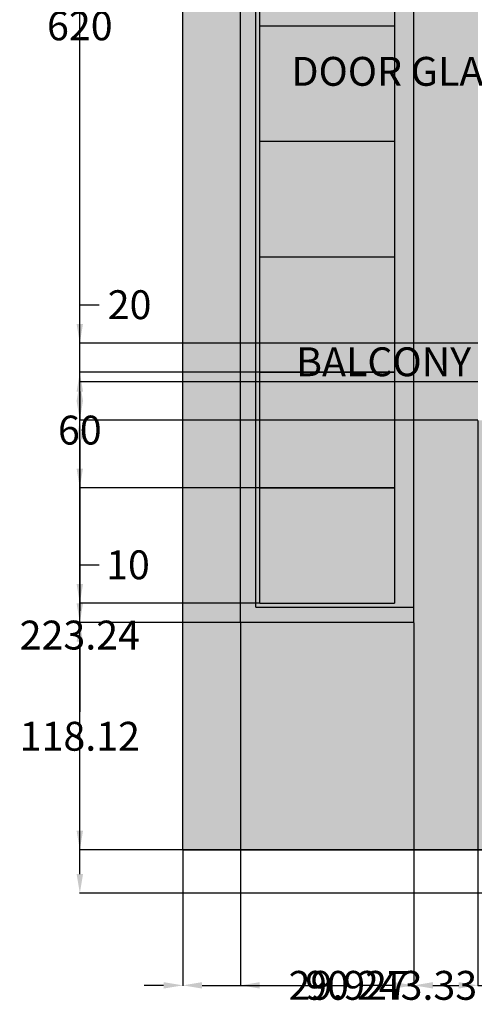
# Model space of a CAD drawing. Units: millimetres. Extents: x 131 to 845, y -20 to 1043.
# Tile 1 of 11: x 131 to 368, y -20 to 492. Entities that reach past the tile are written whole.
import ezdxf

# ---------------------------------------------------------------- set-up
doc = ezdxf.new("R2010")
doc.units = ezdxf.units.MM
doc.header["$MEASUREMENT"] = 0
for name, color, linetype, lineweight in [('A-ANNO-DIMS', 2, 'Continuous', 18), ('A-ELEV', 7, 'Continuous', 25), ('A-ELEV-PATT', 7, 'Continuous', 13), ('A-GLAZ', 4, 'Continuous', 25), ('A-WALL-PATT', 131, 'Continuous', 13)]:
    doc.layers.add(name, color=color, linetype=linetype, lineweight=lineweight)
doc.styles.get("Standard").update_dxf_attribs({"font": 'arial.ttf'})
doc.dimstyles.get("Standard").update_dxf_attribs({"dimtxt": 15, "dimasz": 10, "dimexe": 0.18, "dimexo": 0.0625, "dimgap": 5, "dimtad": 0, "dimtih": 1, "dimtoh": 1, "dimdec": 0, "dimzin": 0, "dimdsep": 46, "dimtxsty": 'Standard', "dimcen": 5, "dimadec": 0, "dimazin": 0, "dimtfac": 1, "dimtdec": 0, "dimtofl": 0, "dimtmove": 0, "dimatfit": 3, "dimfxl": 1, "dimtolj": 1, "dimtzin": 0, "dimarcsym": 0})

# ---------------------------------------------------------------- blocks, each defined once
blk = doc.blocks.new('*U3')
blk.add_line((0, -70), (0, 0))
blk = doc.blocks.new('*U4')
at = {"layer": 'A-GLAZ', "color": 0, "linetype": 'ByBlock', "lineweight": -2, "transparency": 16777216, "rotation": 270}
for p in [(326.16, 488.43), (326.16, 428.43), (326.16, 368.43), (326.16, 308.43), (326.16, 248.43), (326.16, 188.43)]:
    blk.add_blockref('*U3', p, dxfattribs=at)
blk = doc.blocks.new('*D9')
at = {"layer": 'A-ANNO-DIMS', "color": 0, "lineweight": -2, "transparency": 16777216}
for p, q in [((571.05, 313.91), (561.05, 313.91)), ((581.05, 313.22), (581.05, 314.09)), ((586.05, 313.22), (586.05, 314.09)), ((596.05, 313.91), (606.05, 313.91))]:
    blk.add_line(p, q, dxfattribs=at)
at = {"layer": 'A-ANNO-DIMS', "color": 0, "transparency": 16777216}
for points in [[(571.05, 315.58), (571.05, 312.24), (581.05, 313.91)], [(596.05, 315.58), (596.05, 312.24), (586.05, 313.91)]]:
    blk.add_solid(points, dxfattribs=at)
at = {"layer": 'Defpoints', "color": 0, "transparency": 16777216}
for p in [(581.05, 313.91), (581.05, 313.16), (586.05, 313.16)]:
    blk.add_point(p, dxfattribs=at)
at = {"layer": 'A-ANNO-DIMS', "color": 0, "transparency": 16777216, "insert": (409.24, 313.91), "char_height": 15, "attachment_point": 5}
blk.add_mtext('\\A1;BALCONY RAIL PANEL 5 TYP.', dxfattribs=at)
blk = doc.blocks.new('*D11')
at = {"layer": 'A-ANNO-DIMS', "color": 0, "lineweight": -2, "transparency": 16777216}
for p, q in [((554.73, 464.78), (544.73, 464.78)), ((554.75, 454.78), (554.73, 464.78)), ((550.09, 454.77), (554.93, 454.78)), ((554.78, 433.28), (554.76, 444.78)), ((550.13, 423.27), (554.97, 423.28))]:
    blk.add_line(p, q, dxfattribs=at)
at = {"layer": 'A-ANNO-DIMS', "color": 0, "transparency": 16777216}
for points in [[(556.43, 444.78), (553.1, 444.77), (554.75, 454.78)], [(556.45, 433.28), (553.11, 433.27), (554.79, 423.28)]]:
    blk.add_solid(points, dxfattribs=at)
at = {"layer": 'Defpoints', "color": 0, "transparency": 16777216}
for p in [(550.02, 454.77), (554.75, 454.78), (550.07, 423.27)]:
    blk.add_point(p, dxfattribs=at)
at = {"layer": 'A-ANNO-DIMS', "color": 0, "transparency": 16777216, "insert": (399.96, 464.78), "char_height": 15, "attachment_point": 5}
blk.add_mtext('\\A1;DOOR GLASS PANE 32 TYP.', dxfattribs=at)
blk = doc.blocks.new('*D14')
at = {"layer": 'A-ANNO-DIMS', "color": 0, "lineweight": -2, "transparency": 16777216}
for p, q in [((210.52, 985.67), (162.55, 985.67)), ((162.73, 975.67), (162.73, 524.4)), ((162.73, 47.81), (162.73, 499.08)), ((459.5, 37.81), (162.55, 37.81))]:
    blk.add_line(p, q, dxfattribs=at)
at = {"layer": 'A-ANNO-DIMS', "color": 0, "transparency": 16777216}
for points in [[(161.06, 975.67), (164.4, 975.67), (162.73, 985.67)], [(161.06, 47.81), (164.4, 47.81), (162.73, 37.81)]]:
    blk.add_solid(points, dxfattribs=at)
at = {"layer": 'Defpoints', "color": 0, "transparency": 16777216}
for p in [(162.73, 985.67), (210.58, 985.67), (459.56, 37.81)]:
    blk.add_point(p, dxfattribs=at)
at = {"layer": 'A-ANNO-DIMS', "color": 0, "transparency": 16777216, "insert": (162.73, 511.74), "char_height": 15, "attachment_point": 5}
blk.add_mtext('\\A1;947.9', dxfattribs=at)
blk = doc.blocks.new('*D17')
at = {"layer": 'A-ANNO-DIMS', "color": 0, "lineweight": -2, "transparency": 16777216}
for p, q in [((216.17, 960.67), (162.55, 960.67)), ((162.73, 950.67), (162.73, 523.15)), ((162.73, 70.31), (162.73, 497.83)), ((216.17, 60.31), (162.55, 60.31))]:
    blk.add_line(p, q, dxfattribs=at)
at = {"layer": 'A-ANNO-DIMS', "color": 0, "transparency": 16777216}
for points in [[(161.06, 950.67), (164.4, 950.67), (162.73, 960.67)], [(161.06, 70.31), (164.4, 70.31), (162.73, 60.31)]]:
    blk.add_solid(points, dxfattribs=at)
at = {"layer": 'Defpoints', "color": 0, "transparency": 16777216}
for p in [(162.73, 960.67), (216.23, 960.67), (216.23, 60.31)]:
    blk.add_point(p, dxfattribs=at)
at = {"layer": 'A-ANNO-DIMS', "color": 0, "transparency": 16777216, "insert": (162.73, 510.49), "char_height": 15, "attachment_point": 5}
blk.add_mtext('\\A1;900.4', dxfattribs=at)
blk = doc.blocks.new('*D18')
at = {"layer": 'A-ANNO-DIMS', "color": 0, "lineweight": -2, "transparency": 16777216}
for p, q in [((216.23, 60.25), (216.23, -10.22)), ((459.56, 60.25), (459.56, -10.22)), ((226.23, -10.04), (301.63, -10.04)), ((449.56, -10.04), (374.16, -10.04))]:
    blk.add_line(p, q, dxfattribs=at)
at = {"layer": 'A-ANNO-DIMS', "color": 0, "transparency": 16777216}
for points in [[(226.23, -8.37), (226.23, -11.7), (216.23, -10.04)], [(449.56, -8.37), (449.56, -11.7), (459.56, -10.04)]]:
    blk.add_solid(points, dxfattribs=at)
at = {"layer": 'Defpoints', "color": 0, "transparency": 16777216}
for p in [(216.23, 60.31), (459.56, 60.31), (459.56, -10.04)]:
    blk.add_point(p, dxfattribs=at)
at = {"layer": 'A-ANNO-DIMS', "color": 0, "transparency": 16777216, "insert": (337.9, -10.04), "char_height": 15, "attachment_point": 5}
blk.add_mtext('\\A1;243.33', dxfattribs=at)
blk = doc.blocks.new('*D25')
at = {"layer": 'A-ANNO-DIMS', "color": 0, "lineweight": -2, "transparency": 16777216}
for p, q in [((246.16, 178.37), (246.16, -10.22)), ((216.23, 60.25), (216.23, -10.22)), ((206.23, -10.04), (196.23, -10.04)), ((256.16, -10.04), (266.16, -10.04))]:
    blk.add_line(p, q, dxfattribs=at)
at = {"layer": 'A-ANNO-DIMS', "color": 0, "transparency": 16777216}
for points in [[(206.23, -8.37), (206.23, -11.7), (216.23, -10.04)], [(256.16, -8.37), (256.16, -11.7), (246.16, -10.04)]]:
    blk.add_solid(points, dxfattribs=at)
at = {"layer": 'Defpoints', "color": 0, "transparency": 16777216}
for p in [(246.16, 178.43), (216.23, 60.31), (246.16, -10.04)]:
    blk.add_point(p, dxfattribs=at)
at = {"layer": 'A-ANNO-DIMS', "color": 0, "transparency": 16777216, "insert": (302.42, -10.04), "char_height": 15, "attachment_point": 5}
blk.add_mtext('\\A1;29.927', dxfattribs=at)
blk = doc.blocks.new('*D26')
at = {"layer": 'A-ANNO-DIMS', "color": 0, "lineweight": -2, "transparency": 16777216}
for p, q in [((246.16, 178.37), (246.16, -10.22)), ((336.16, 178.37), (336.16, -10.22)), ((256.16, -10.04), (275.44, -10.04)), ((326.16, -10.04), (306.88, -10.04))]:
    blk.add_line(p, q, dxfattribs=at)
at = {"layer": 'A-ANNO-DIMS', "color": 0, "transparency": 16777216}
for points in [[(256.16, -8.37), (256.16, -11.7), (246.16, -10.04)], [(326.16, -8.37), (326.16, -11.7), (336.16, -10.04)]]:
    blk.add_solid(points, dxfattribs=at)
at = {"layer": 'Defpoints', "color": 0, "transparency": 16777216}
for p in [(246.16, 178.43), (336.16, 178.43), (336.16, -10.04)]:
    blk.add_point(p, dxfattribs=at)
at = {"layer": 'A-ANNO-DIMS', "color": 0, "transparency": 16777216, "insert": (291.16, -10.04), "char_height": 15, "attachment_point": 5}
blk.add_mtext('\\A1;90', dxfattribs=at)
blk = doc.blocks.new('*D27')
at = {"layer": 'A-ANNO-DIMS', "color": 0, "lineweight": -2, "transparency": 16777216}
for p, q in [((246.1, 178.43), (162.55, 178.43)), ((162.73, 168.43), (162.73, 132.03)), ((162.73, 70.31), (162.73, 106.71)), ((216.17, 60.31), (162.55, 60.31))]:
    blk.add_line(p, q, dxfattribs=at)
at = {"layer": 'A-ANNO-DIMS', "color": 0, "transparency": 16777216}
for points in [[(161.06, 168.43), (164.4, 168.43), (162.73, 178.43)], [(161.06, 70.31), (164.4, 70.31), (162.73, 60.31)]]:
    blk.add_solid(points, dxfattribs=at)
at = {"layer": 'Defpoints', "color": 0, "transparency": 16777216}
for p in [(246.16, 178.43), (162.73, 60.31), (216.23, 60.31)]:
    blk.add_point(p, dxfattribs=at)
at = {"layer": 'A-ANNO-DIMS', "color": 0, "transparency": 16777216, "insert": (162.73, 119.37), "char_height": 15, "attachment_point": 5}
blk.add_mtext('\\A1;118.12', dxfattribs=at)
blk = doc.blocks.new('*D28')
at = {"layer": 'A-ANNO-DIMS', "color": 0, "lineweight": -2, "transparency": 16777216}
for p, q in [((246.1, 798.43), (162.55, 798.43)), ((162.73, 788.43), (162.73, 501.09)), ((162.73, 188.43), (162.73, 475.77)), ((246.1, 178.43), (162.55, 178.43))]:
    blk.add_line(p, q, dxfattribs=at)
at = {"layer": 'A-ANNO-DIMS', "color": 0, "transparency": 16777216}
for points in [[(161.06, 788.43), (164.4, 788.43), (162.73, 798.43)], [(161.06, 188.43), (164.4, 188.43), (162.73, 178.43)]]:
    blk.add_solid(points, dxfattribs=at)
at = {"layer": 'Defpoints', "color": 0, "transparency": 16777216}
for p in [(162.73, 798.43), (246.16, 798.43), (246.16, 178.43)]:
    blk.add_point(p, dxfattribs=at)
at = {"layer": 'A-ANNO-DIMS', "color": 0, "transparency": 16777216, "insert": (162.73, 488.43), "char_height": 15, "attachment_point": 5}
blk.add_mtext('\\A1;620', dxfattribs=at)
blk = doc.blocks.new('*D29')
at = {"layer": 'A-ANNO-DIMS', "color": 0, "lineweight": -2, "transparency": 16777216}
for p, q in [((326.1, 308.43), (162.55, 308.43)), ((162.73, 298.43), (162.73, 291.09)), ((162.73, 258.43), (162.73, 265.77)), ((326.1, 248.43), (162.55, 248.43))]:
    blk.add_line(p, q, dxfattribs=at)
at = {"layer": 'A-ANNO-DIMS', "color": 0, "transparency": 16777216}
for points in [[(161.06, 298.43), (164.4, 298.43), (162.73, 308.43)], [(161.06, 258.43), (164.4, 258.43), (162.73, 248.43)]]:
    blk.add_solid(points, dxfattribs=at)
at = {"layer": 'Defpoints', "color": 0, "transparency": 16777216}
for p in [(162.73, 308.43), (326.16, 308.43), (326.16, 248.43)]:
    blk.add_point(p, dxfattribs=at)
at = {"layer": 'A-ANNO-DIMS', "color": 0, "transparency": 16777216, "insert": (162.73, 278.43), "char_height": 15, "attachment_point": 5}
blk.add_mtext('\\A1;60', dxfattribs=at)
blk = doc.blocks.new('*D32')
at = {"layer": 'A-ANNO-DIMS', "color": 0, "lineweight": -2, "transparency": 16777216}
for p, q in [((162.73, 198.43), (162.73, 208.43)), ((162.73, 208.43), (172.73, 208.43)), ((256.1, 188.43), (162.55, 188.43)), ((246.1, 178.43), (162.55, 178.43)), ((162.73, 168.43), (162.73, 158.43))]:
    blk.add_line(p, q, dxfattribs=at)
at = {"layer": 'A-ANNO-DIMS', "color": 0, "transparency": 16777216}
for points in [[(161.06, 198.43), (164.4, 198.43), (162.73, 188.43)], [(161.06, 168.43), (164.4, 168.43), (162.73, 178.43)]]:
    blk.add_solid(points, dxfattribs=at)
at = {"layer": 'Defpoints', "color": 0, "transparency": 16777216}
for p in [(162.73, 188.43), (256.16, 188.43), (246.16, 178.43)]:
    blk.add_point(p, dxfattribs=at)
at = {"layer": 'A-ANNO-DIMS', "color": 0, "transparency": 16777216, "insert": (187.74, 208.43), "char_height": 15, "attachment_point": 5}
blk.add_mtext('\\A1;10', dxfattribs=at)
blk = doc.blocks.new('*D33')
at = {"layer": 'A-ANNO-DIMS', "color": 0, "lineweight": -2, "transparency": 16777216}
for p, q in [((369.56, 283.49), (369.56, -10.22)), ((336.16, 178.37), (336.16, -10.22)), ((346.16, -10.04), (359.56, -10.04)), ((369.56, -10.04), (379.56, -10.04))]:
    blk.add_line(p, q, dxfattribs=at)
at = {"layer": 'A-ANNO-DIMS', "color": 0, "transparency": 16777216}
for points in [[(346.16, -8.37), (346.16, -11.7), (336.16, -10.04)], [(359.56, -8.37), (359.56, -11.7), (369.56, -10.04)]]:
    blk.add_solid(points, dxfattribs=at)
at = {"layer": 'Defpoints', "color": 0, "transparency": 16777216}
for p in [(369.56, 283.56), (336.16, 178.43), (369.56, -10.04)]:
    blk.add_point(p, dxfattribs=at)
at = {"layer": 'A-ANNO-DIMS', "color": 0, "transparency": 16777216, "insert": (404, -10.04), "char_height": 15, "attachment_point": 5}
blk.add_mtext('\\A1;33.4', dxfattribs=at)
blk = doc.blocks.new('*D35')
at = {"layer": 'A-ANNO-DIMS', "color": 0, "lineweight": -2, "transparency": 16777216}
for p, q in [((369.5, 763.56), (162.55, 763.56)), ((162.73, 753.56), (162.73, 536.21)), ((162.73, 293.56), (162.73, 510.9)), ((369.5, 283.56), (162.55, 283.56))]:
    blk.add_line(p, q, dxfattribs=at)
at = {"layer": 'A-ANNO-DIMS', "color": 0, "transparency": 16777216}
for points in [[(161.06, 753.56), (164.4, 753.56), (162.73, 763.56)], [(161.06, 293.56), (164.4, 293.56), (162.73, 283.56)]]:
    blk.add_solid(points, dxfattribs=at)
at = {"layer": 'Defpoints', "color": 0, "transparency": 16777216}
for p in [(162.73, 763.56), (369.56, 763.56), (369.56, 283.56)]:
    blk.add_point(p, dxfattribs=at)
at = {"layer": 'A-ANNO-DIMS', "color": 0, "transparency": 16777216, "insert": (162.73, 523.56), "char_height": 15, "attachment_point": 5}
blk.add_mtext('\\A1;480', dxfattribs=at)
blk = doc.blocks.new('*D36')
at = {"layer": 'A-ANNO-DIMS', "color": 0, "lineweight": -2, "transparency": 16777216}
for p, q in [((162.73, 333.56), (162.73, 343.56)), ((162.73, 343.56), (172.73, 343.56)), ((369.5, 323.56), (162.55, 323.56)), ((369.5, 303.56), (162.55, 303.56)), ((162.73, 293.56), (162.73, 283.56))]:
    blk.add_line(p, q, dxfattribs=at)
at = {"layer": 'A-ANNO-DIMS', "color": 0, "transparency": 16777216}
for points in [[(161.06, 333.56), (164.4, 333.56), (162.73, 323.56)], [(161.06, 293.56), (164.4, 293.56), (162.73, 303.56)]]:
    blk.add_solid(points, dxfattribs=at)
at = {"layer": 'Defpoints', "color": 0, "transparency": 16777216}
for p in [(162.73, 323.56), (369.56, 323.56), (369.56, 303.56)]:
    blk.add_point(p, dxfattribs=at)
at = {"layer": 'A-ANNO-DIMS', "color": 0, "transparency": 16777216, "insert": (188.58, 343.56), "char_height": 15, "attachment_point": 5}
blk.add_mtext('\\A1;20', dxfattribs=at)
blk = doc.blocks.new('*D37')
at = {"layer": 'A-ANNO-DIMS', "color": 0, "lineweight": -2, "transparency": 16777216}
for p, q in [((369.5, 283.56), (162.55, 283.56)), ((162.73, 273.56), (162.73, 184.6)), ((162.73, 70.31), (162.73, 159.27)), ((216.17, 60.31), (162.55, 60.31))]:
    blk.add_line(p, q, dxfattribs=at)
at = {"layer": 'A-ANNO-DIMS', "color": 0, "transparency": 16777216}
for points in [[(161.06, 273.56), (164.4, 273.56), (162.73, 283.56)], [(161.06, 70.31), (164.4, 70.31), (162.73, 60.31)]]:
    blk.add_solid(points, dxfattribs=at)
at = {"layer": 'Defpoints', "color": 0, "transparency": 16777216}
for p in [(369.56, 283.56), (162.73, 60.31), (216.23, 60.31)]:
    blk.add_point(p, dxfattribs=at)
at = {"layer": 'A-ANNO-DIMS', "color": 0, "transparency": 16777216, "insert": (162.73, 171.93), "char_height": 15, "attachment_point": 5}
blk.add_mtext('\\A1;223.24', dxfattribs=at)
blk = doc.blocks.new('*D50')
at = {"layer": 'A-ANNO-DIMS', "color": 0, "lineweight": -2, "transparency": 16777216}
for p, q in [((720.6, 488.6), (768.56, 488.6)), ((768.38, 478.6), (768.38, 287.12)), ((768.38, 70.31), (768.38, 261.79)), ((216.3, 60.31), (768.56, 60.31))]:
    blk.add_line(p, q, dxfattribs=at)
at = {"layer": 'A-ANNO-DIMS', "color": 0, "transparency": 16777216}
for points in [[(766.72, 478.6), (770.05, 478.6), (768.38, 488.6)], [(766.72, 70.31), (770.05, 70.31), (768.38, 60.31)]]:
    blk.add_solid(points, dxfattribs=at)
at = {"layer": 'Defpoints', "color": 0, "transparency": 16777216}
for p in [(720.53, 488.6), (768.38, 488.6), (216.23, 60.31)]:
    blk.add_point(p, dxfattribs=at)
at = {"layer": 'A-ANNO-DIMS', "color": 0, "transparency": 16777216, "insert": (768.38, 274.45), "char_height": 15, "attachment_point": 5}
blk.add_mtext('\\A1;428.3', dxfattribs=at)

msp = doc.modelspace()

# ---------------------------------------------------------------- hatches: boundary and pattern name
at = {"layer": 'A-ELEV-PATT'}
h = msp.add_hatch(color=256, dxfattribs=at)
h.set_gradient(color1=(199, 200, 202), color2=(99, 100, 102), name='SPHERICAL')
h.paths.add_polyline_path([(255.6595, 927.8345), (255.6595, 860.8345), (326.6595, 860.8345), (326.6595, 927.8345)])
h.paths.add_polyline_path([(336.1595, 798.4332), (246.1595, 798.4332), (246.1595, 178.4332), (336.1595, 178.4332), (336.1595, 186.4332), (254.1595, 186.4332), (254.1595, 788.4332), (256.1595, 788.4332), (326.1595, 788.4332), (326.1595, 188.4332), (256.1595, 188.4332), (256.1595, 788.4332), (254.1595, 788.4332), (254.1595, 186.4332), (336.1595, 186.4332), (336.1595, 188.4332)])
h = msp.add_hatch(color=256, dxfattribs=at)
h.set_gradient(color1=(199, 200, 202), color2=(255, 255, 0), name='INVCYLINDER')
h.paths.add_polyline_path([(326.1595, 728.4332), (326.1595, 788.4332), (256.1595, 788.4332), (256.1595, 728.4332)])
h.paths.add_polyline_path([(326.1595, 668.4332), (326.1595, 728.4332), (256.1595, 728.4332), (256.1595, 668.4332)])
h.paths.add_polyline_path([(326.1595, 608.4332), (326.1595, 668.4332), (256.1595, 668.4332), (256.1595, 608.4332)])
h.paths.add_polyline_path([(326.1595, 548.4332), (326.1595, 608.4332), (256.1595, 608.4332), (256.1595, 548.4332)])
h.paths.add_polyline_path([(326.1595, 488.4332), (326.1595, 548.4332), (256.1595, 548.4332), (256.1595, 488.4332)])
h.paths.add_polyline_path([(326.1595, 428.4332), (326.1595, 488.4332), (256.1595, 488.4332), (256.1595, 428.4332)])
h.paths.add_polyline_path([(326.1595, 368.4332), (326.1595, 428.4332), (256.1595, 428.4332), (256.1595, 368.4332)])
h.paths.add_polyline_path([(256.1595, 368.4332), (256.1595, 308.4332), (326.1595, 308.4332), (326.1595, 368.4332)])
h.paths.add_polyline_path([(256.1595, 308.4332), (256.1595, 248.4332), (326.1595, 248.4332), (326.1595, 308.4332)])
h.paths.add_polyline_path([(256.1595, 248.4332), (256.1595, 188.4332), (326.1595, 188.4332), (326.1595, 248.4332)])
at = {"layer": 'A-WALL-PATT'}
h = msp.add_hatch(color=256, dxfattribs=at)
h.dxf.hatch_style = 1
h.paths.add_polyline_path([(449.5586, 833.5953), (451.6297, 835.6663), (451.6297, 885.6663), (466.6297, 885.6663), (466.6297, 891.3345), (330.6595, 891.3345), (330.6595, 856.8345), (292.1595, 856.8345), (292.1595, 798.4332), (336.1595, 798.4332), (336.1595, 178.4332), (246.1595, 178.4332), (246.1595, 798.4332), (290.1595, 798.4332), (290.1595, 856.8345), (259.6595, 856.8345), (255.6595, 860.8345), (255.6595, 927.8345), (290.1595, 927.8345), (290.1595, 960.6663), (216.2327, 960.6663), (216.2327, 60.3131), (459.5586, 60.3131), (459.5586, 97.8131), (459.5586, 252.07), (459.5586, 283.5561), (369.5586, 283.5561), (369.5586, 763.5561), (439.5586, 763.5561), (439.5586, 778.6714), (439.5586, 793.5953), (439.5586, 796.5953), (441.5586, 798.5953), (444.5586, 798.5953), (444.5586, 813.5953), (444.5586, 816.5953), (446.5586, 818.5953), (449.5586, 818.5953)])
h.paths.add_polyline_path([(466.6297, 960.6663), (292.1595, 960.6663), (292.1595, 927.8345), (326.6595, 927.8345), (330.6595, 923.8345), (330.6595, 893.3345), (466.6297, 893.3345)], flags=17)
h.paths.add_polyline_path([(720.5349, 813.5953), (720.5349, 818.5953), (710.5349, 818.5953), (449.5586, 818.5953), (446.5586, 818.5953), (444.5586, 816.5953), (444.5586, 813.5953), (444.5586, 798.5953), (705.5349, 798.5953), (705.5349, 513.5953), (705.5349, 498.5953), (680.5349, 498.5953), (680.5349, 488.5953), (705.5349, 488.5953), (720.5349, 488.5953), (720.5349, 513.5953)])
h.paths.add_polyline_path([(680.5349, 498.5953), (412.6606, 498.5953), (412.6606, 488.5953), (680.5349, 488.5953)])

# ---------------------------------------------------------------- linework, layer by layer
at = {"layer": 'A-ELEV'}
for p, q in [((216.2327, 60.3131), (216.2327, 960.6663)), ((246.1595, 178.4332), (246.1595, 798.4332)), ((336.1595, 798.4332), (336.1595, 178.4332)), ((254.1595, 186.4332), (254.1595, 788.4332)), ((256.1595, 188.4332), (256.1595, 788.4332)), ((326.1595, 788.4332), (326.1595, 188.4332)), ((254.1595, 186.4332), (336.1595, 186.4332)), ((336.1595, 188.4332), (336.1595, 178.4332)), ((336.1595, 178.4332), (246.1595, 178.4332)), ((459.5586, 60.3131), (216.2327, 60.3131))]:
    msp.add_line(p, q, dxfattribs=at)

# ---------------------------------------------------------------- block references
at = {"layer": 'A-GLAZ'}
msp.add_blockref('*U4', (0, 0), dxfattribs=at)

# ---------------------------------------------------------------- dimensions: what is measured, and where the dimension line sits
at = {"layer": 'A-ANNO-DIMS'}
for base, p1, p2, override, picture, middle in [((162.7317, 985.6663), (459.5586, 37.8131), (210.5817, 985.6663), {"dimdec": 1, "dimlfac": 1, "dimrnd": 0, "dimzin": 0, "dimdsep": 46, "dimlunit": 2}, '*D14', (162.7317, 511.7397)), ((162.7317, 960.6663), (216.2327, 60.3131), (216.2327, 960.6663), {"dimdec": 1, "dimlfac": 1, "dimrnd": 0, "dimzin": 0, "dimdsep": 46, "dimlunit": 2}, '*D17', (162.7317, 510.4897)), ((162.7317, 798.4332), (246.1595, 178.4332), (246.1595, 798.4332), {"dimdec": 0, "dimlfac": 1, "dimrnd": 0, "dimzin": 0, "dimdsep": 46, "dimlunit": 2}, '*D28', (162.7317, 488.4332)), ((162.7317, 763.5561), (369.5586, 283.5561), (369.5586, 763.5561), {"dimdec": 0, "dimlfac": 1, "dimrnd": 0, "dimzin": 0, "dimdsep": 46, "dimlunit": 2}, '*D35', (162.7317, 523.5561)), ((768.3849, 488.5953), (216.2327, 60.3131), (720.5349, 488.5953), {"dimdec": 1, "dimlfac": 1, "dimrnd": 0, "dimzin": 0, "dimdsep": 46, "dimlunit": 2}, '*D50', (768.3849, 274.4542)), ((162.7317, 323.5561), (369.5586, 303.5561), (369.5586, 323.5561), {"dimdec": 0, "dimlfac": 1, "dimrnd": 0, "dimzin": 0, "dimdsep": 46, "dimlunit": 2}, '*D36', (188.5775, 343.5561)), ((162.7317, 308.4332), (326.1595, 248.4332), (326.1595, 308.4332), {"dimdec": 0, "dimlfac": 1, "dimrnd": 0, "dimzin": 0, "dimdsep": 46, "dimlunit": 2}, '*D29', (162.7317, 278.4332)), ((162.7317, 60.3131), (369.5586, 283.5561), (216.2327, 60.3131), {"dimdec": 2, "dimlfac": 1, "dimrnd": 0, "dimzin": 0, "dimdsep": 46, "dimlunit": 2}, '*D37', (162.7317, 171.9346)), ((162.7317, 188.4332), (246.1595, 178.4332), (256.1595, 188.4332), {"dimdec": 0, "dimlfac": 1, "dimrnd": 0, "dimzin": 0, "dimdsep": 46, "dimlunit": 2}, '*D32', (187.7436, 208.4332)), ((162.7317, 60.3131), (246.1595, 178.4332), (216.2327, 60.3131), {"dimdec": 2, "dimlfac": 1, "dimrnd": 0, "dimzin": 0, "dimdsep": 46, "dimlunit": 2}, '*D27', (162.7317, 119.3731))]:
    dim = msp.add_linear_dim(base=base, p1=p1, p2=p2, angle=90, dimstyle='Standard', override=override, dxfattribs=at)
    dim.commit()
    dim.dimension.update_dxf_attribs({"geometry": picture, "text_midpoint": middle})
for base, p1, p2, angle, text, picture, middle in [((554.7491, 454.7757), (550.0694, 423.2689), (550.0241, 454.7689), 90.082356, 'DOOR GLASS PANE <> TYP.', '*D11', (399.9615, 464.7756)), ((581.0467, 313.9096), (586.0467, 313.1596), (581.0467, 313.1596), 180, 'BALCONY RAIL PANEL <> TYP.', '*D9', (409.2391, 313.9096))]:
    dim = msp.add_linear_dim(base=base, p1=p1, p2=p2, angle=angle, text=text, dimstyle='Standard', override={"dimdec": 0, "dimrnd": 0, "dimzin": 0, "dimlunit": 2}, dxfattribs=at)
    dim.commit()
    dim.dimension.update_dxf_attribs({"geometry": picture, "text_midpoint": middle})
for base, p1, p2, override, picture, middle in [((369.5586, -10.0369), (336.1595, 178.4332), (369.5586, 283.5561), {"dimdec": 1, "dimlfac": 1, "dimrnd": 0, "dimzin": 0, "dimdsep": 46, "dimlunit": 2}, '*D33', (404.0044, -10.0369)), ((246.1595, -10.0369), (216.2327, 60.3131), (246.1595, 178.4332), {"dimdec": 3, "dimlfac": 1, "dimrnd": 0, "dimzin": 0, "dimdsep": 46, "dimlunit": 2}, '*D25', (302.4232, -10.0369)), ((336.1595, -10.0369), (246.1595, 178.4332), (336.1595, 178.4332), {"dimdec": 0, "dimlfac": 1, "dimrnd": 0, "dimzin": 0, "dimdsep": 46, "dimlunit": 2}, '*D26', (291.1595, -10.0369)), ((459.5586, -10.0369), (216.2327, 60.3131), (459.5586, 60.3131), {"dimdec": 2, "dimlfac": 1, "dimrnd": 0, "dimzin": 0, "dimdsep": 46, "dimlunit": 2}, '*D18', (337.8956, -10.0369))]:
    dim = msp.add_linear_dim(base=base, p1=p1, p2=p2, dimstyle='Standard', override=override, dxfattribs=at)
    dim.commit()
    dim.dimension.update_dxf_attribs({"geometry": picture, "text_midpoint": middle})

doc.saveas('drawing.dxf')
